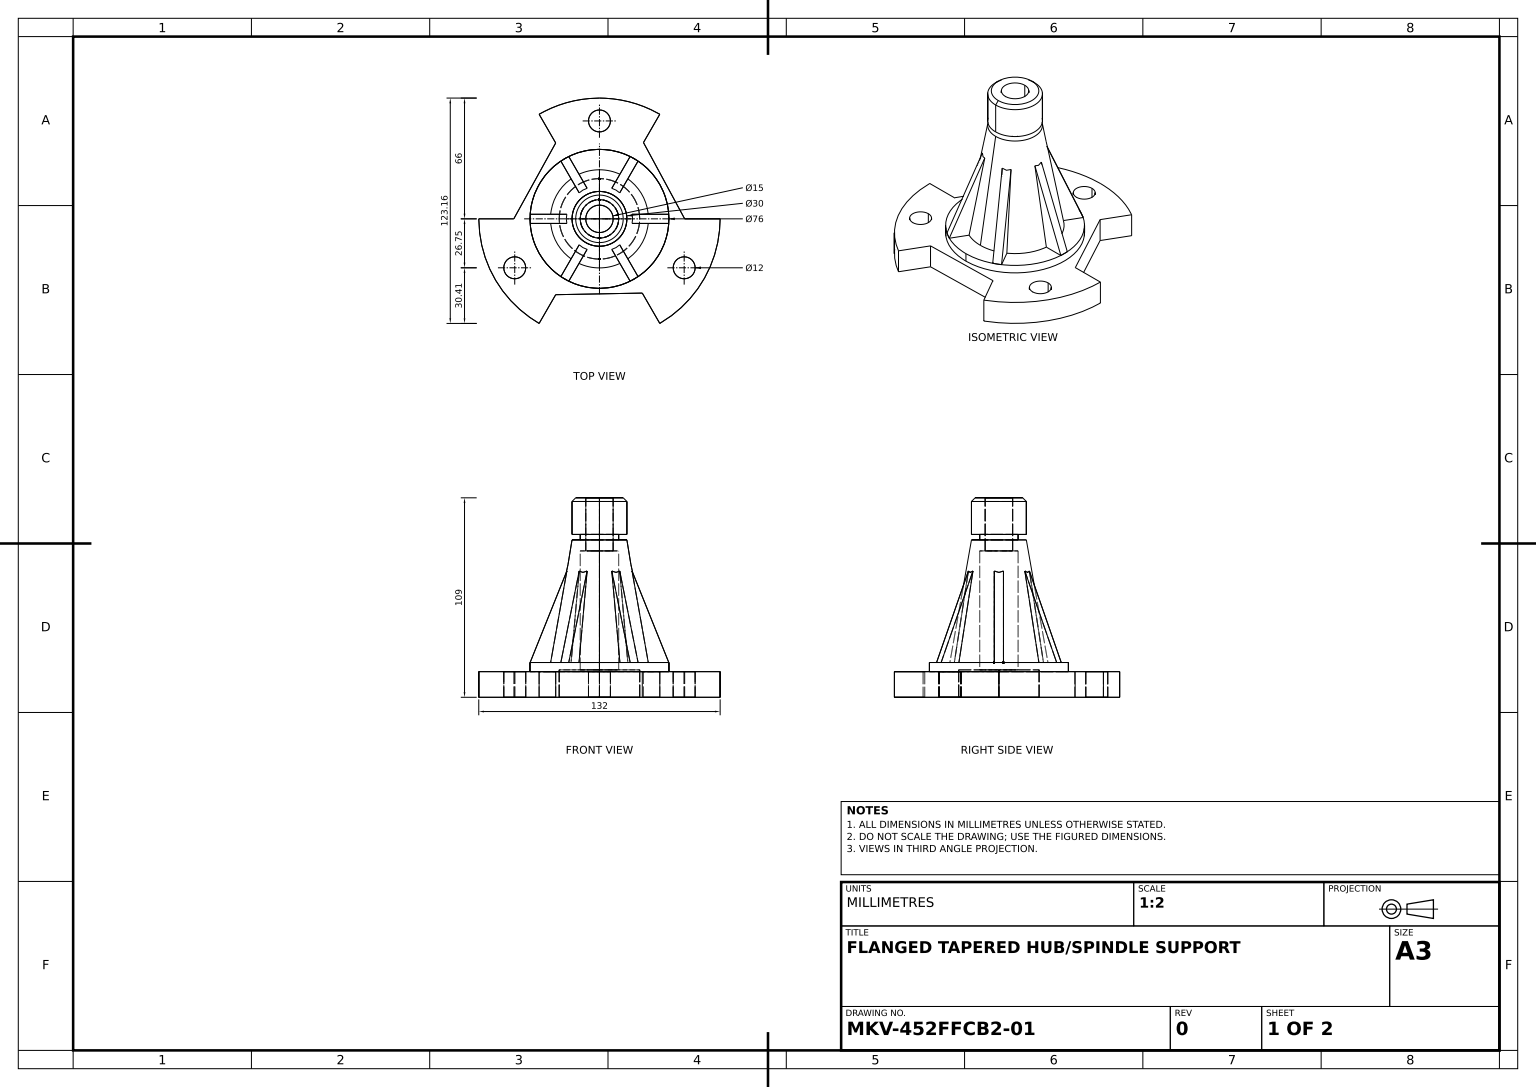
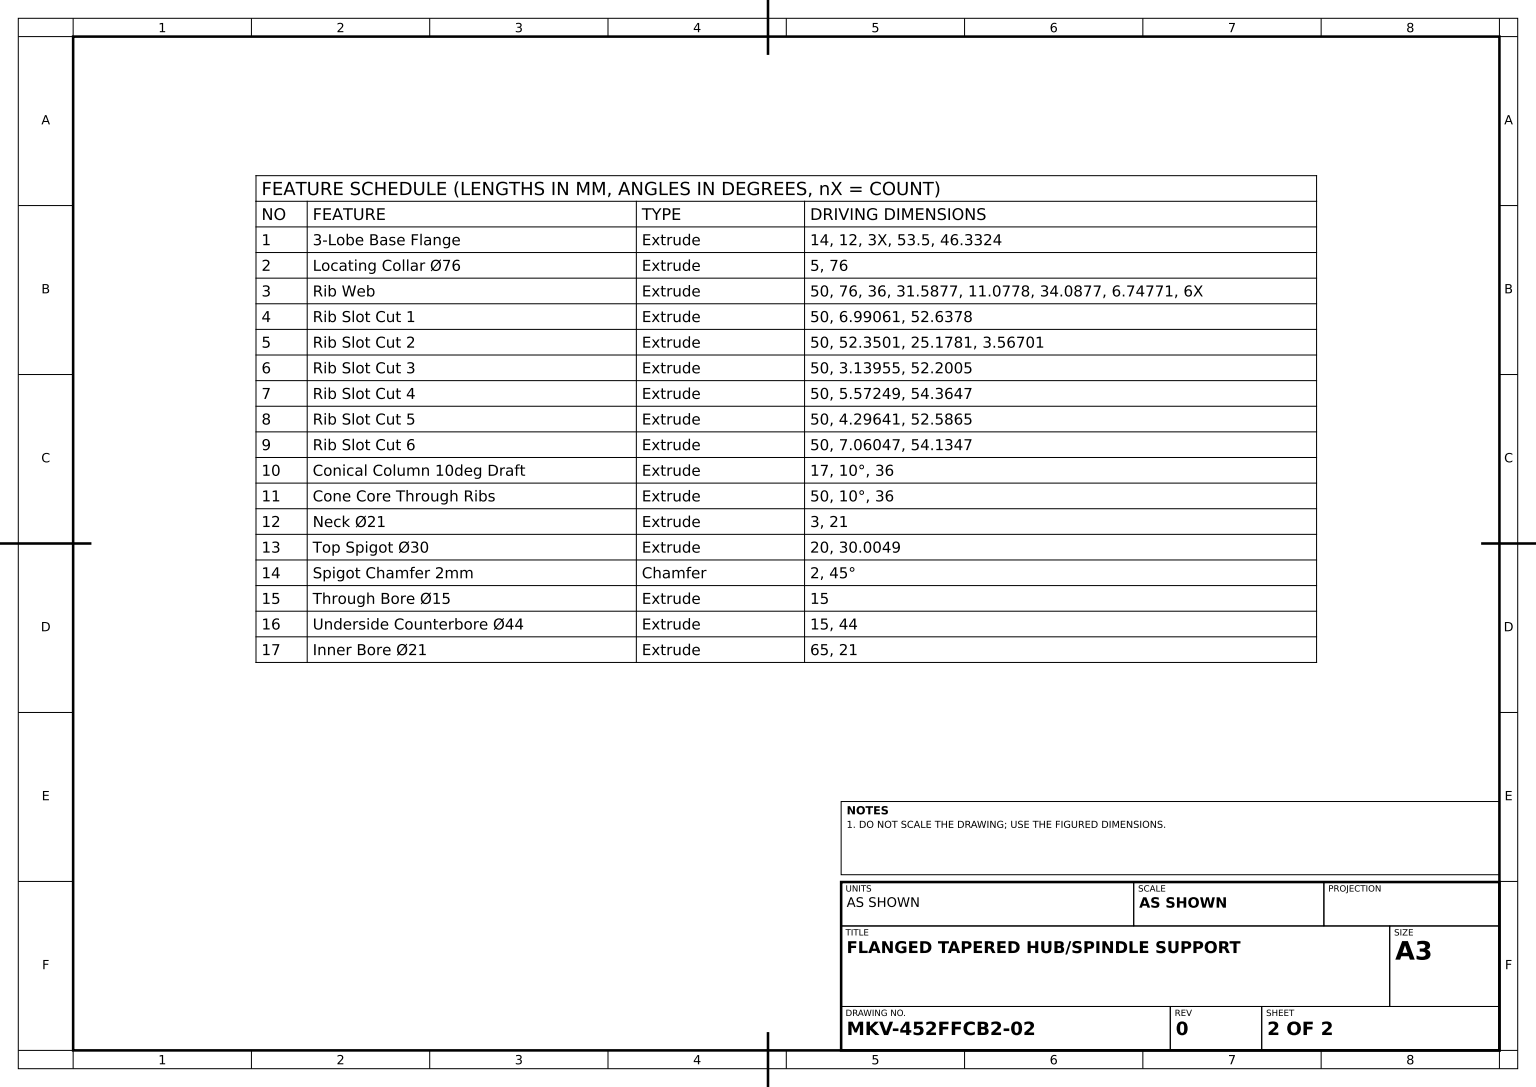
from build123d import *

# Parameters (mm, degrees)
BASE_FLANGE_SKETCH_R             = 6
F_3_LOBE_BASE_FLANGE_DEPTH       = 14
LOCATING_COLLAR_SKETCH_R         = 38
LOCATING_COLLAR_76_DEPTH         = 5
RIB_WEB_DEPTH                    = 50
RIB_SLOT_CUT_1_DEPTH             = 50
RIB_SLOT_CUT_2_DEPTH             = 50
RIB_SLOT_CUT_3_DEPTH             = 50
RIB_SLOT_CUT_4_DEPTH             = 50
RIB_SLOT_CUT_5_DEPTH             = 50
RIB_SLOT_CUT_6_DEPTH             = 50
CONE_BASE_SKETCH_36_R            = 18
CONICAL_COLUMN_10DEG_DRAFT_DEPTH = 17
CONICAL_COLUMN_10DEG_DRAFT_TAPER = 10
SKETCH10_2_R                     = 18
CONE_CORE_THROUGH_RIBS_DEPTH     = 50
CONE_CORE_THROUGH_RIBS_DRAFT     = 10
NECK_SKETCH_R                    = 10.5
NECK_21_DEPTH                    = 3
TOP_SPIGOT_SKETCH_R              = 15.002441328
TOP_SPIGOT_30_DEPTH              = 20
SPIGOT_CHAMFER_2MM_SIZE          = 2
THROUGH_BORE_SKETCH_R            = 7.5
THROUGH_BORE_15_DEPTH            = 144.502613217
UNDERSIDE_COUNTERBORE_SKETCH_R   = 22
UNDERSIDE_COUNTERBORE_44_DEPTH   = 15
INNER_BORE_SKETCH_R              = 10.5
INNER_BORE_21_DEPTH              = 65


with BuildPart() as part:
    # Base Flange Sketch → 3-Lobe Base Flange (new body)
    with BuildSketch(Plane(origin=(0, 0, 0), x_dir=(1, 0, 0), z_dir=(0, 1, 0))):
        with BuildLine():
            Line((33, -57.15767665), (23.422856537, -40.56957758))
            Line((23.422856537, -40.56957758), (-23.933636252, -41.454273999))
            Line((-23.933636252, -41.454273999), (-33, -57.15767665))
            ThreePointArc((-33, -57.15767665), (-57.15767665, -33), (-66, 0))
            Line((-66, 0), (-46.845713073, 0))
            Line((-46.845713073, 0), (-23.933636252, 41.454273999))
            Line((-23.933636252, 41.454273999), (-33, 57.15767665))
            ThreePointArc((-33, 57.15767665), (0, 66), (33, 57.15767665))
            Line((33, 57.15767665), (24.073038277, 41.695725388))
            Line((24.073038277, 41.695725388), (46.60222479, 0))
            Line((46.60222479, 0), (66, 0))
            ThreePointArc((66, 0), (57.15767665, -33), (33, -57.15767665))
        make_face()
        with Locations(Location((0, 53.5, 0), (0, 0, 270))):
            Circle(BASE_FLANGE_SKETCH_R, mode=Mode.SUBTRACT)
        with Locations(Location((46.332359102, -26.75, 0), (0, 0, 270))):
            Circle(BASE_FLANGE_SKETCH_R, mode=Mode.SUBTRACT)
        with Locations(Location((-46.332359102, -26.75, 0), (0, 0, 270))):
            Circle(BASE_FLANGE_SKETCH_R, mode=Mode.SUBTRACT)
    extrude(amount=F_3_LOBE_BASE_FLANGE_DEPTH)

    # Locating Collar Sketch → Locating Collar _76 (add)
    with BuildSketch(Plane(origin=(0, 14, 0), x_dir=(1, 0, 0), z_dir=(0, 1, 0))):
        with Locations(Location((0, 0, 0), (0, 0, 270))):
            Circle(LOCATING_COLLAR_SKETCH_R)
    extrude(amount=LOCATING_COLLAR_76_DEPTH)

    # Rib Web Sketch → Rib Web (add)
    with BuildSketch(Plane(origin=(0, 19, 0), x_dir=(1, 0, 0), z_dir=(0, 1, 0))):
        with BuildLine():
            Line((37.917673979, 2.5), (17.82554347, 2.5))
            ThreePointArc((17.82554347, 2.5), (15.588457268, 9), (11.077835244, 14.187373481))
            Line((11.077835244, 14.187373481), (21.123900499, 31.587668918))
            ThreePointArc((21.123900499, 31.587668918), (19, 32.908965344), (16.79377348, 34.087668918))
            Line((16.79377348, 34.087668918), (6.747708226, 16.687373481))
            ThreePointArc((6.747708226, 16.687373481), (0, 18), (-6.747708226, 16.687373481))
            Line((-6.747708226, 16.687373481), (-16.79377348, 34.087668918))
            ThreePointArc((-16.79377348, 34.087668918), (-19, 32.908965344), (-21.123900499, 31.587668918))
            Line((-21.123900499, 31.587668918), (-11.077835244, 14.187373481))
            ThreePointArc((-11.077835244, 14.187373481), (-15.588457268, 9), (-17.82554347, 2.5))
            Line((-17.82554347, 2.5), (-37.917673979, 2.5))
            ThreePointArc((-37.917673979, 2.5), (-38, 0), (-37.917673979, -2.5))
            Line((-37.917673979, -2.5), (-17.82554347, -2.5))
            ThreePointArc((-17.82554347, -2.5), (-15.588457268, -9), (-11.077835244, -14.187373481))
            Line((-11.077835244, -14.187373481), (-21.123900499, -31.587668918))
            ThreePointArc((-21.123900499, -31.587668918), (-19, -32.908965344), (-16.79377348, -34.087668918))
            Line((-16.79377348, -34.087668918), (-6.747708226, -16.687373481))
            ThreePointArc((-6.747708226, -16.687373481), (0, -18), (6.747708226, -16.687373481))
            Line((6.747708226, -16.687373481), (16.79377348, -34.087668918))
            ThreePointArc((16.79377348, -34.087668918), (19, -32.908965344), (21.123900499, -31.587668918))
            Line((21.123900499, -31.587668918), (11.077835244, -14.187373481))
            ThreePointArc((11.077835244, -14.187373481), (15.588457268, -9), (17.82554347, -2.5))
            Line((17.82554347, -2.5), (37.917673979, -2.5))
            ThreePointArc((37.917673979, -2.5), (37.979412918, -1.250677574), (38, 0))
            ThreePointArc((38, 0), (37.979412918, 1.250677574), (37.917673979, 2.5))
        make_face()
    extrude(amount=RIB_WEB_DEPTH)

    # Rib Slot 1 Sketch → Rib Slot Cut 1 (cut)
    with BuildSketch(Plane(origin=(-2.165063509, 0, 1.25), x_dir=(0.5000000000000031, 0, 0.8660254037844369), z_dir=(-0.8660254037844369, 0, 0.5000000000000031))):
        Polygon((17.82554347, 69), (37.917673979, 19), (44.908281954, 19), (44.908281954, 71.637843916), align=None)
    extrude(amount=-RIB_SLOT_CUT_1_DEPTH, mode=Mode.SUBTRACT)

    # Rib Slot 2 Sketch → Rib Slot Cut 2 (cut)
    with BuildSketch(Plane.XY.offset(2.5)):
        Polygon((37.917673979, 19), (41.484682242, 19), (43.003646089, 71.350074734), (17.82554347, 69), align=None)
    extrude(amount=-RIB_SLOT_CUT_2_DEPTH, mode=Mode.SUBTRACT)

    # Rib Slot 3 Sketch → Rib Slot Cut 3 (cut)
    with BuildSketch(Plane(origin=(2.165063509, 0, 1.25), x_dir=(0.49999999999999784, 0, -0.86602540378444), z_dir=(0.86602540378444, 0, 0.49999999999999784))):
        Polygon((17.82554347, 69), (37.917673979, 19), (41.057228015, 19), (41.057228015, 71.20053138), align=None)
    extrude(amount=-RIB_SLOT_CUT_3_DEPTH, mode=Mode.SUBTRACT)

    # Rib Slot 4 Sketch → Rib Slot Cut 4 (cut)
    with BuildSketch(Plane(origin=(2.165063509, 0, -1.25), x_dir=(-0.5000000000000029, 0, -0.866025403784437), z_dir=(0.866025403784437, 0, -0.5000000000000029))):
        Polygon((17.82554347, 69), (37.917673979, 19), (43.490166386, 19), (43.490166386, 73.364655625), align=None)
    extrude(amount=-RIB_SLOT_CUT_4_DEPTH, mode=Mode.SUBTRACT)

    # Rib Slot 5 Sketch → Rib Slot Cut 5 (cut)
    with BuildSketch(Plane(origin=(0, 0, -2.5), x_dir=(-1, 0, 0), z_dir=(0, 0, -1))):
        Polygon((17.82554347, 69), (37.917673979, 19), (42.214088477, 19), (42.214088477, 71.586453607), align=None)
    extrude(amount=-RIB_SLOT_CUT_5_DEPTH, mode=Mode.SUBTRACT)

    # Rib Slot 6 Sketch → Rib Slot Cut 6 (cut)
    with BuildSketch(Plane(origin=(-2.165063509, 0, -1.25), x_dir=(-0.4999999999999972, 0, 0.8660254037844403), z_dir=(-0.8660254037844403, 0, -0.4999999999999972))):
        Polygon((17.82554347, 69), (37.917673979, 19), (44.978143034, 19), (44.978143034, 73.134659176), align=None)
    extrude(amount=-RIB_SLOT_CUT_6_DEPTH, mode=Mode.SUBTRACT)

    # Cone Base Sketch _36 → Conical Column 10deg Draft (add)
    with BuildSketch(Plane(origin=(0, 69, 0), x_dir=(1, 0, 0), z_dir=(0, 1, 0))):
        Circle(CONE_BASE_SKETCH_36_R)
    extrude(amount=CONICAL_COLUMN_10DEG_DRAFT_DEPTH, taper=CONICAL_COLUMN_10DEG_DRAFT_TAPER)


with BuildPart() as cone_core_through_ribs_tool:
    # Sketch10_2 → Cone Core Through Ribs (with draft: the straight prism first)
    with BuildSketch(Plane(origin=(0, 69, 0), x_dir=(1, 0, 0), z_dir=(0, 1, 0))):
        Circle(SKETCH10_2_R)
    extrude(amount=-CONE_CORE_THROUGH_RIBS_DEPTH)
    # Cone Core Through Ribs: the draft: its side faces are tilted about the plane it starts from
    cone_core_through_ribs_sides = [cone_core_through_ribs_tool.faces().sort_by_distance(p)[0] for p in [
        (-18, 44, 0),
    ]]
    draft(cone_core_through_ribs_sides, Plane(origin=(0, 69, 0), x_dir=(1, 0, 0), z_dir=(0, 1, 0)), CONE_CORE_THROUGH_RIBS_DRAFT)


with BuildPart() as part_1:
    add(part.part)

    # Cone Core Through Ribs: add cone_core_through_ribs_tool
    add(cone_core_through_ribs_tool.part)

    # Neck Sketch → Neck _21 (add)
    with BuildSketch(Plane(origin=(0, 86, 0), x_dir=(1, 0, 0), z_dir=(0, 1, 0))):
        with Locations(Location((0, 0, 0), (0, 0, 270))):
            Circle(NECK_SKETCH_R)
    extrude(amount=NECK_21_DEPTH)

    # Top Spigot Sketch → Top Spigot _30 (add)
    with BuildSketch(Plane(origin=(0, 89, 0), x_dir=(1, 0, 0), z_dir=(0, 1, 0))):
        with Locations(Location((0, 0, 0), (0, 0, 270))):
            Circle(TOP_SPIGOT_SKETCH_R)
    extrude(amount=TOP_SPIGOT_30_DEPTH)

    # Spigot Chamfer 2mm
    spigot_chamfer_2mm_edges = [part_1.edges().sort_by_distance(p)[0] for p in [
        (0, 109, -15.002441328),
    ]]
    chamfer(spigot_chamfer_2mm_edges, length=SPIGOT_CHAMFER_2MM_SIZE)

    # Through Bore Sketch → Through Bore _15 (cut, through all)
    with BuildSketch(Plane(origin=(0, 109, 0), x_dir=(1, 0, 0), z_dir=(0, 1, 0))):
        with Locations(Location((0, 0, 0), (0, 0, 270))):
            Circle(THROUGH_BORE_SKETCH_R)
    extrude(amount=-THROUGH_BORE_15_DEPTH, mode=Mode.SUBTRACT)

    # Underside Counterbore Sketch → Underside Counterbore _44 (cut)
    with BuildSketch(Plane.XZ):
        with Locations(Location((0, 0, 0), (0, 0, 270))):
            Circle(UNDERSIDE_COUNTERBORE_SKETCH_R)
    extrude(amount=-UNDERSIDE_COUNTERBORE_44_DEPTH, mode=Mode.SUBTRACT)

    # Inner Bore Sketch → Inner Bore _21 (cut)
    with BuildSketch(Plane.XZ.offset(-15)):
        with Locations(Location((0, 0, 0), (0, 0, 90))):
            Circle(INNER_BORE_SKETCH_R)
    extrude(amount=-INNER_BORE_21_DEPTH, mode=Mode.SUBTRACT)


solid = part_1.part
